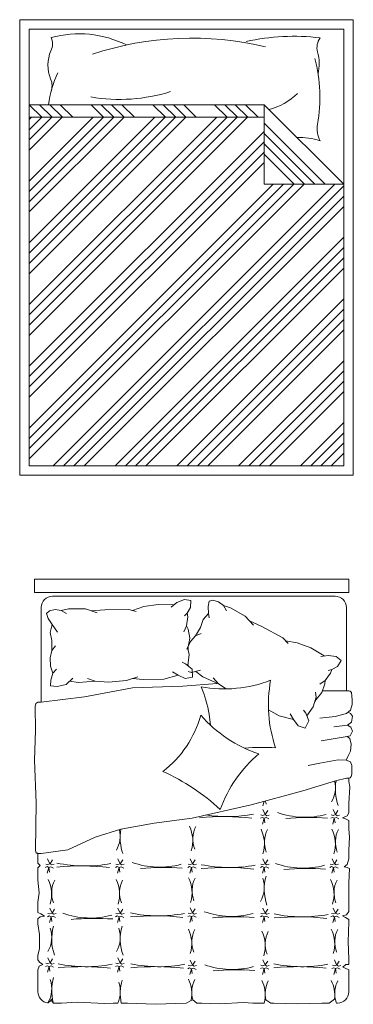
# Model space of a CAD drawing. Units: inches. Extents: x 1994 to 3075, y 3517 to 3950.
# Tile 25 of 58: x 1994.3682 to 1994.4307, y 3553.7004 to 3553.8849. Entities that reach past the tile are written whole.
import ezdxf

# ---------------------------------------------------------------- set-up
doc = ezdxf.new("R2010")
doc.units = ezdxf.units.IN
doc.layers.add('A-FURN-REFR', color=8, linetype='Continuous', lineweight=13)
doc.layers.add('A-FURN-REFR-PATT', color=8, linetype='Continuous', lineweight=13)

msp = doc.modelspace()

# ---------------------------------------------------------------- hatches: boundary and pattern name
at = {"layer": 'A-FURN-REFR-PATT'}
h = msp.add_hatch(dxfattribs=at)
h.set_pattern_fill('ANSI34', color=256, scale=0.0004294917680744, style=0)
h.set_pattern_definition([(45, (1992.977044442859, 3553.850180684118), (-0.005785419118799, 0.005785419118799), []), (45, (1992.978972916732, 3553.850180684118), (-0.005785419118799, 0.005785419118799), []), (45, (1992.980901390605, 3553.850180684118), (-0.005785419118799, 0.005785419118799), []), (45, (1992.982829868772, 3553.850180684118), (-0.005785419118799, 0.005785419118799), [])])
h.paths.add_polyline_path([(1994.370029690871, 3553.801315221915), (1994.428938814508, 3553.801315221915), (1994.428938814508, 3553.854071563733), (1994.414015178144, 3553.854071563733), (1994.414015178144, 3553.866638836461), (1994.370029690871, 3553.866638836461)])

# ---------------------------------------------------------------- linework, layer by layer
at = {"layer": 'A-FURN-REFR'}
for p, q in [((1994.368240141838, 3553.884922930949), (1994.430728363541, 3553.884922930949)), ((1994.368240141838, 3553.799525672881), (1994.368240141838, 3553.884922930949)), ((1994.430728363541, 3553.799525672881), (1994.430728363541, 3553.884922930949)), ((1994.370029690871, 3553.801315221915), (1994.370029690871, 3553.883133381916)), ((1994.370029690871, 3553.883133381916), (1994.428938814508, 3553.883133381916)), ((1994.428938814508, 3553.883133381916), (1994.428938814508, 3553.801315221915)), ((1994.370029690871, 3553.868995200097), (1994.414015178144, 3553.868995200097)), ((1994.372386054507, 3553.866638836461), (1994.370029690871, 3553.868995200097)), ((1994.370029690871, 3553.868995200097), (1994.414015178144, 3553.868995200097)), ((1994.374314532675, 3553.866638836461), (1994.371958169039, 3553.868995200097)), ((1994.376243006548, 3553.866638836461), (1994.373886642911, 3553.868995200097)), ((1994.37817148042, 3553.866638836461), (1994.375815116784, 3553.868995200097)), ((1994.383956892745, 3553.866638836461), (1994.381600529109, 3553.868995200097)), ((1994.385885370913, 3553.866638836461), (1994.383529007276, 3553.868995200097)), ((1994.387813844785, 3553.866638836461), (1994.385457481149, 3553.868995200097)), ((1994.389742318658, 3553.866638836461), (1994.387385955021, 3553.868995200097)), ((1994.395527730983, 3553.866638836461), (1994.393171367346, 3553.868995200097)), ((1994.39745620915, 3553.866638836461), (1994.395099845514, 3553.868995200097)), ((1994.399384683022, 3553.866638836461), (1994.397028319387, 3553.868995200097)), ((1994.401313156896, 3553.866638836461), (1994.398956793259, 3553.868995200097)), ((1994.407098569221, 3553.866638836461), (1994.404742205584, 3553.868995200097)), ((1994.409027047388, 3553.866638836461), (1994.406670683751, 3553.868995200097)), ((1994.41095552126, 3553.866638836461), (1994.408599157624, 3553.868995200097)), ((1994.412883995133, 3553.866638836461), (1994.410527631497, 3553.868995200097)), ((1994.428938814508, 3553.854071563733), (1994.414015178144, 3553.868995200097)), ((1994.414015178144, 3553.868995200097), (1994.414015178144, 3553.854071563733)), ((1994.414015178144, 3553.866638836461), (1994.370029690871, 3553.866638836461)), ((1994.42545126786, 3553.854071563733), (1994.414015178144, 3553.86550765345)), ((1994.423522793988, 3553.854071563733), (1994.414015178144, 3553.863579179578)), ((1994.421594320115, 3553.854071563733), (1994.414015178144, 3553.861650705704)), ((1994.419665841948, 3553.854071563733), (1994.414015178144, 3553.859722227537)), ((1994.414015178144, 3553.854071563733), (1994.428938814508, 3553.854071563733)), ((1994.428938814508, 3553.801315221915), (1994.370029690871, 3553.801315221915)), ((1994.368240141838, 3553.799525672881), (1994.430728363541, 3553.799525672881)), ((1994.374369662702, 3553.776879347694), (1994.427307661648, 3553.776879347694)), ((1994.406405658198, 3553.77509977936), (1994.407753984843, 3553.774702339899)), ((1994.406405658198, 3553.77509977936), (1994.406968598159, 3553.774142304752)), ((1994.372252142744, 3553.757002402463), (1994.372252142744, 3553.774761827737)), ((1994.403633649272, 3553.773621406152), (1994.402579506154, 3553.772507359423)), ((1994.407753984843, 3553.774702339899), (1994.410494828313, 3553.773116088013)), ((1994.410494828313, 3553.773116088013), (1994.412065912074, 3553.771412908928)), ((1994.429425181607, 3553.76268197533), (1994.429425181607, 3553.774761827737)), ((1994.402579506154, 3553.772507359423), (1994.402115540643, 3553.771021464581)), ((1994.402115540643, 3553.771021464581), (1994.401170657182, 3553.769426673137)), ((1994.399767832714, 3553.766897611043), (1994.399767832714, 3553.767096424024)), ((1994.399767832714, 3553.763831583339), (1994.399767832714, 3553.763991882089)), ((1994.429425181607, 3553.76268197533), (1994.429425181607, 3553.759155137558)), ((1994.398783393365, 3553.759994420633), (1994.405228269321, 3553.7605222814)), ((1994.393114474107, 3553.759840917956), (1994.398783393365, 3553.759994420633)), ((1994.429425181607, 3553.759155137558), (1994.429893852388, 3553.759155137558)), ((1994.371652995319, 3553.757002402463), (1994.372252613397, 3553.757002402463)), ((1994.423521127195, 3553.757099635416), (1994.42361858113, 3553.757272925152)), ((1994.403701135297, 3553.754744186191), (1994.403958917441, 3553.752696826246)), ((1994.429474495267, 3553.754878016059), (1994.427309408632, 3553.754311432808)), ((1994.430203898, 3553.755507485811), (1994.429474495267, 3553.754878016059)), ((1994.427309408632, 3553.754311432808), (1994.42447417688, 3553.754002387236)), ((1994.427103209532, 3553.752354144484), (1994.429629144984, 3553.752663190056)), ((1994.429629144984, 3553.752663190056), (1994.430247740718, 3553.75230263659)), ((1994.430557038585, 3553.751581530554), (1994.430144641951, 3553.75070590173)), ((1994.430247740718, 3553.75230263659), (1994.430557038585, 3553.751581530554)), ((1994.429216746784, 3553.750499871051), (1994.42468037598, 3553.749778765014)), ((1994.430144641951, 3553.75070590173), (1994.429216746784, 3553.750499871051)), ((1994.424459448261, 3553.74558966953), (1994.422300593145, 3553.745123270979)), ((1994.427901946281, 3553.746172667719), (1994.424459448261, 3553.74558966953)), ((1994.429418979945, 3553.7461143679), (1994.427901946281, 3553.746172667719)), ((1994.430177496776, 3553.745822868806), (1994.429418979945, 3553.7461143679)), ((1994.430462438404, 3553.745117864219), (1994.430177496776, 3553.745822868806)), ((1994.429425181607, 3553.742779105069), (1994.429893852388, 3553.742779105069)), ((1994.429893852388, 3553.742779105069), (1994.429893852388, 3553.74212236867)), ((1994.429893852388, 3553.738038066713), (1994.429893852388, 3553.736243449602)), ((1994.429893852388, 3553.734820132314), (1994.429893852388, 3553.733211165113)), ((1994.429893852388, 3553.72918874646), (1994.429893852388, 3553.727631897226)), ((1994.371652995319, 3553.726829779951), (1994.371652995319, 3553.728685223678)), ((1994.372252142744, 3553.728620422557), (1994.371652995319, 3553.728620422557)), ((1994.371652995319, 3553.723611844897), (1994.371652995319, 3553.725963413047)), ((1994.371652995319, 3553.717547275919), (1994.371652995319, 3553.719527543594)), ((1994.429893852388, 3553.718596926409), (1994.429893852388, 3553.717762449974)), ((1994.371652995319, 3553.715443241637), (1994.371652995319, 3553.716371491844)), ((1994.429893852388, 3553.716245358913), (1994.429893852388, 3553.715812175133)), ((1994.371652995319, 3553.708697955665), (1994.371652995319, 3553.709564322569)), ((1994.429893852388, 3553.708881239251), (1994.429893852388, 3553.707829221784)), ((1994.371652995319, 3553.705851321087), (1994.371652995319, 3553.706841454597)), ((1994.429893852388, 3553.706839088273), (1994.429893852388, 3553.702720755229)), ((1994.376058946635, 3553.700603235272), (1994.374596919452, 3553.700603235272)), ((1994.38661782809, 3553.700603235272), (1994.385720626736, 3553.700603235272)), ((1994.388420073799, 3553.700603235272), (1994.387271361502, 3553.700603235272)), ((1994.40235518889, 3553.700603235272), (1994.401426181978, 3553.700603235272)), ((1994.414013487327, 3553.700603235272), (1994.411893001706, 3553.700603235272)), ((1994.415856768486, 3553.700603235272), (1994.415299363426, 3553.700603235272)), ((1994.426199720931, 3553.700603235272), (1994.424837176243, 3553.700603235272)), ((1994.427560077345, 3553.700603235272), (1994.42777633243, 3553.700603235272))]:
    msp.add_line(p, q, dxfattribs=at)
msp.add_lwpolyline([(1994.370993535893, 3553.780030975446), (1994.429881082485, 3553.780030975446), (1994.429881082485, 3553.777551780742), (1994.370993535893, 3553.777551780742)], close=True, dxfattribs=at)
for points in [[(1994.389379899846, 3553.774159662139), (1994.391495423462, 3553.77490501664), (1994.394172619542, 3553.775298872562), (1994.39712136546, 3553.775228739967)], [(1994.399084448324, 3553.773206591587), (1994.399594702442, 3553.773700236123), (1994.400226090622, 3553.774741015109), (1994.400300586028, 3553.776056433098), (1994.39913322836, 3553.776216902284), (1994.397700281661, 3553.77566724495), (1994.39659355446, 3553.774828945053)], [(1994.406405658198, 3553.77509977936), (1994.405466822385, 3553.775811861941), (1994.404429321561, 3553.776144065447), (1994.403742598781, 3553.775963909912), (1994.40351379457, 3553.774962775242), (1994.403633649272, 3553.773621406152), (1994.403727248118, 3553.772789354132)], [(1994.376026324964, 3553.774197287111), (1994.374858967296, 3553.774357756296), (1994.373791819769, 3553.774138751078), (1994.373281565651, 3553.773645106542), (1994.37357287003, 3553.772660340705), (1994.374334848873, 3553.771549924374), (1994.375346156134, 3553.770146197392)], [(1994.376026324964, 3553.774197287111), (1994.377396372352, 3553.774511791517), (1994.380562898609, 3553.774472683474), (1994.382767152017, 3553.773758267566)], [(1994.376026324964, 3553.774197287111), (1994.376986329604, 3553.773638672652)], [(1994.381656957109, 3553.774118090488), (1994.384200098715, 3553.774307924899), (1994.388673773663, 3553.774348168371), (1994.39008579642, 3553.773971217203)], [(1994.398958777189, 3553.770191613156), (1994.39950861096, 3553.771304552722), (1994.39971356891, 3553.773013448286), (1994.399594702442, 3553.773700236123)], [(1994.374334848873, 3553.771549924374), (1994.373962116957, 3553.770062178177), (1994.374286068838, 3553.768539613678), (1994.374244220954, 3553.766686396676)], [(1994.399747945956, 3553.766984136998), (1994.400109875452, 3553.769027707226), (1994.399776595705, 3553.770703928636), (1994.39950861096, 3553.771304552722)], [(1994.411274619573, 3553.772270732598), (1994.413584330142, 3553.771189601976), (1994.417503409388, 3553.769031777853), (1994.418549385725, 3553.768011075178)], [(1994.402233276213, 3553.769852220113), (1994.401170657182, 3553.769426673137), (1994.400219416478, 3553.768348255874), (1994.399547527007, 3553.766963226722)], [(1994.374961828736, 3553.767578186171), (1994.374244220954, 3553.766686396676), (1994.373943716215, 3553.765280146495), (1994.374036994797, 3553.763743578786), (1994.374423846009, 3553.762456166863)], [(1994.4180264826, 3553.768521343527), (1994.420235776237, 3553.768134025673), (1994.422762338659, 3553.767165013974), (1994.42529815245, 3553.765658471747)], [(1994.399751169989, 3553.76384533263), (1994.399988868261, 3553.765935900162), (1994.399747945956, 3553.766984136998)], [(1994.426018003793, 3553.762933661213), (1994.426704726573, 3553.763113816748), (1994.427765226226, 3553.763711489248), (1994.428474948234, 3553.764821520203), (1994.427536112421, 3553.765533602784), (1994.426017694354, 3553.765756909736), (1994.424642129816, 3553.765568723605)], [(1994.396869108781, 3553.762662051774), (1994.397910668443, 3553.762031276771), (1994.39925979189, 3553.761419172675), (1994.400634503815, 3553.761656848839), (1994.400541225232, 3553.763193416547), (1994.399322563715, 3553.76419899818), (1994.398688779206, 3553.764468969762)], [(1994.375150781636, 3553.763194299799), (1994.374423846009, 3553.762456166863), (1994.374041786226, 3553.761122077577), (1994.37403019013, 3553.760041812517), (1994.375269775589, 3553.759962839385), (1994.376947387375, 3553.760296014735), (1994.378184576506, 3553.761527792171)], [(1994.389350455634, 3553.761407307046), (1994.391398246481, 3553.761250377201), (1994.395252128075, 3553.761330107378), (1994.397910668443, 3553.762031276771)], [(1994.399768886277, 3553.762736315327), (1994.400394365444, 3553.762531641508), (1994.402076517846, 3553.762998841562)], [(1994.401232126903, 3553.7627643209), (1994.402574387931, 3553.761730739291), (1994.405449609264, 3553.760421493173)], [(1994.424430587178, 3553.760367341538), (1994.425455373825, 3553.761067887029), (1994.426471684252, 3553.762456931638), (1994.426704726573, 3553.763113816748)], [(1994.377563544014, 3553.760909476191), (1994.379240127958, 3553.760666531976), (1994.382387998502, 3553.760934737404)], [(1994.380966647265, 3553.761465345445), (1994.382387998502, 3553.760934737404), (1994.384867168785, 3553.760776791455), (1994.388245712014, 3553.761059000053), (1994.390366014664, 3553.761727495645)], [(1994.404470821382, 3553.761580699158), (1994.405449609264, 3553.760421493173), (1994.406887043621, 3553.759488094975)], [(1994.423546206662, 3553.757184801398), (1994.424863387386, 3553.758788611605), (1994.425394541905, 3553.760413009488), (1994.425455373825, 3553.761067887029)], [(1994.372252613397, 3553.757002402463), (1994.380392096975, 3553.757998261552), (1994.389362140071, 3553.759658026504), (1994.393114474107, 3553.759840917956)], [(1994.422010441024, 3553.754447370638), (1994.423242376189, 3553.756153040251), (1994.423771411884, 3553.75794956339), (1994.423622200712, 3553.75887743124)], [(1994.42498323605, 3553.759155137558), (1994.429425652259, 3553.759155137558)], [(1994.429893852388, 3553.759155137558), (1994.430137944852, 3553.759073556183), (1994.430412507876, 3553.758799217356), (1994.430490954223, 3553.757420990779), (1994.430542340634, 3553.756552727357)], [(1994.371652995319, 3553.757002402463), (1994.371239196245, 3553.756726399039), (1994.37112370645, 3553.756207118058), (1994.371181451348, 3553.751706682294), (1994.371008216138, 3553.746109986878), (1994.371296941142, 3553.738147677905), (1994.371181451348, 3553.729262202644), (1994.371296941142, 3553.728685223678), (1994.371652995319, 3553.728685223678)], [(1994.430542340634, 3553.756552727357), (1994.430203898, 3553.755507485811)], [(1994.414840307951, 3553.755539734691), (1994.416856067451, 3553.754460380967), (1994.419517007735, 3553.753768375036)], [(1994.418918354215, 3553.754828722901), (1994.419517007735, 3553.753768375036), (1994.42039289265, 3553.752573539853), (1994.421707625421, 3553.752106848761), (1994.422379514892, 3553.753491877914), (1994.421810217842, 3553.754965727019), (1994.421390131811, 3553.755511707957)], [(1994.429745537723, 3553.755111923912), (1994.430196191334, 3553.754878016059), (1994.430557038585, 3553.754362940702), (1994.430402388869, 3553.7532812812), (1994.429629144984, 3553.752663190056)], [(1994.429610551763, 3553.750587311863), (1994.430060801397, 3553.750195353428), (1994.430352539844, 3553.749145957585), (1994.430235844465, 3553.747805061751), (1994.429710716826, 3553.74681396483), (1994.429418979945, 3553.7461143679)], [(1994.429893852388, 3553.742779105069), (1994.430158810292, 3553.74282672715), (1994.430322240182, 3553.743048811095), (1994.430479132875, 3553.74351257445), (1994.430462438404, 3553.745117864219)], [(1994.372252142744, 3553.728620422557), (1994.377258563176, 3553.729322034035), (1994.382359210027, 3553.731683821727), (1994.387211044382, 3553.733175476649), (1994.39343134463, 3553.734294218187), (1994.400522487398, 3553.735288655111), (1994.411594622811, 3553.737774746955), (1994.421298292331, 3553.740385143414), (1994.427394186735, 3553.742249712182), (1994.429425181607, 3553.742779105069)], [(1994.429893852388, 3553.738038066713), (1994.430062065296, 3553.741133415707), (1994.429893852388, 3553.74212236867)], [(1994.413431986664, 3553.735883925484), (1994.413793317279, 3553.735789742057), (1994.414233198661, 3553.735946714436), (1994.414688790035, 3553.73666878738)], [(1994.414987280684, 3553.735836833771), (1994.414547399302, 3553.735711255868), (1994.414216404339, 3553.735920096887), (1994.413793317279, 3553.736888548247)], [(1994.426594833989, 3553.735883925484), (1994.426956164605, 3553.735789742057), (1994.427396045987, 3553.735946714436), (1994.427851637361, 3553.73666878738)], [(1994.42815012801, 3553.735836833771), (1994.427710246627, 3553.735711255868), (1994.427379251665, 3553.735920096887), (1994.426956164605, 3553.736888548247)], [(1994.429893852388, 3553.734820132314), (1994.429256925668, 3553.735130729378), (1994.428699520608, 3553.735316379942), (1994.429566595019, 3553.735687679764), (1994.429893852388, 3553.736243449602)], [(1994.413337726714, 3553.735256036432), (1994.413683347338, 3553.735397311573), (1994.41401325797, 3553.735240339193), (1994.414154648704, 3553.734376991573)], [(1994.414877309934, 3553.735130458528), (1994.414390299386, 3553.735381614335), (1994.41401325797, 3553.735240339193), (1994.413714767321, 3553.734157230241)], [(1994.42650057404, 3553.735256036432), (1994.426846194664, 3553.735397311573), (1994.427176105296, 3553.735240339193), (1994.427317496029, 3553.734376991573)], [(1994.42804015726, 3553.735130458528), (1994.427553146712, 3553.735381614335), (1994.427176105296, 3553.735240339193), (1994.426877614647, 3553.734157230241)], [(1994.429893852388, 3553.72918874646), (1994.430000131654, 3553.731789028371), (1994.429893852388, 3553.733211165113)], [(1994.373116485853, 3553.726657353991), (1994.373477816468, 3553.726563170563), (1994.373917697851, 3553.726720142942), (1994.374373289225, 3553.727442215887)], [(1994.374671779874, 3553.726610262277), (1994.374231898491, 3553.726484684374), (1994.373900903528, 3553.726693525393), (1994.373477816468, 3553.727661976754)], [(1994.386273964593, 3553.726657353991), (1994.386635295209, 3553.726563170563), (1994.387075176591, 3553.726720142942), (1994.387530767965, 3553.727442215887)], [(1994.387829258614, 3553.726610262277), (1994.387389377232, 3553.726484684374), (1994.387058382269, 3553.726693525393), (1994.386635295209, 3553.727661976754)], [(1994.399821387241, 3553.726657353991), (1994.400182717856, 3553.726563170563), (1994.400622599238, 3553.726720142942), (1994.401078190612, 3553.727442215887)], [(1994.401376681262, 3553.726610262277), (1994.400936799879, 3553.726484684374), (1994.400605804916, 3553.726693525393), (1994.400182717856, 3553.727661976754)], [(1994.413431986664, 3553.726657353991), (1994.413793317279, 3553.726563170563), (1994.414233198661, 3553.726720142942), (1994.414688790035, 3553.727442215887)], [(1994.414987280684, 3553.726610262277), (1994.414547399302, 3553.726484684374), (1994.414216404339, 3553.726693525393), (1994.413793317279, 3553.727661976754)], [(1994.426418264744, 3553.726657353991), (1994.426779595359, 3553.726563170563), (1994.427219476742, 3553.726720142942), (1994.427675068116, 3553.727442215887)], [(1994.427973558765, 3553.726610262277), (1994.427533677383, 3553.726484684374), (1994.42720268242, 3553.726693525393), (1994.426779595359, 3553.727661976754)], [(1994.429893852388, 3553.718596926409), (1994.429871042563, 3553.723146302614), (1994.429994909847, 3553.725807286627), (1994.429561373212, 3553.725992936538), (1994.429003968152, 3553.726116703799), (1994.429561373212, 3553.726549886925), (1994.429893852388, 3553.727631897226)], [(1994.371652995319, 3553.726829779951), (1994.372103251061, 3553.726371100662), (1994.371652995319, 3553.725963413047)], [(1994.373022225904, 3553.726029464939), (1994.373367846527, 3553.72617074008), (1994.37369775716, 3553.7260137677), (1994.373839147893, 3553.725150420079)], [(1994.374561809123, 3553.725903887035), (1994.374074798576, 3553.726155042841), (1994.37369775716, 3553.7260137677), (1994.37339926651, 3553.724930658748)], [(1994.386179704644, 3553.726029464939), (1994.386525325268, 3553.72617074008), (1994.3868552359, 3553.7260137677), (1994.386996626634, 3553.725150420079)], [(1994.387719287864, 3553.725903887035), (1994.387232277317, 3553.726155042841), (1994.3868552359, 3553.7260137677), (1994.386556745251, 3553.724930658748)], [(1994.399727127292, 3553.726029464939), (1994.400072747915, 3553.72617074008), (1994.400402658547, 3553.7260137677), (1994.400544049281, 3553.725150420079)], [(1994.401266710511, 3553.725903887035), (1994.400779699964, 3553.726155042841), (1994.400402658547, 3553.7260137677), (1994.400104167898, 3553.724930658748)], [(1994.413337726714, 3553.726029464939), (1994.413683347338, 3553.72617074008), (1994.41401325797, 3553.7260137677), (1994.414154648704, 3553.725150420079)], [(1994.414877309934, 3553.725903887035), (1994.414390299386, 3553.726155042841), (1994.41401325797, 3553.7260137677), (1994.413714767321, 3553.724930658748)], [(1994.426324004795, 3553.726029464939), (1994.426669625418, 3553.72617074008), (1994.426999536051, 3553.7260137677), (1994.427140926784, 3553.725150420079)], [(1994.427863588014, 3553.725903887035), (1994.427376577467, 3553.726155042841), (1994.426999536051, 3553.7260137677), (1994.426701045401, 3553.724930658748)], [(1994.371652995319, 3553.723611844897), (1994.371855516493, 3553.72123478189), (1994.371652995319, 3553.719527543594)], [(1994.373521320336, 3553.717410971881), (1994.373882650952, 3553.717316788453), (1994.374322532334, 3553.717473760833), (1994.374778123708, 3553.718195833777)], [(1994.375076614357, 3553.717363880168), (1994.374636732975, 3553.717238302264), (1994.374305738012, 3553.717447143283), (1994.373882650952, 3553.718415594644)], [(1994.386273964593, 3553.717410971881), (1994.386635295209, 3553.717316788453), (1994.387075176591, 3553.717473760833), (1994.387530767965, 3553.718195833777)], [(1994.387829258614, 3553.717363880168), (1994.387389377232, 3553.717238302264), (1994.387058382269, 3553.717447143283), (1994.386635295209, 3553.718415594644)], [(1994.399821387241, 3553.717456636363), (1994.400182717856, 3553.717362452935), (1994.400622599238, 3553.717519425314), (1994.401078190612, 3553.718241498258)], [(1994.401376681262, 3553.717409544649), (1994.400936799879, 3553.717283966745), (1994.400605804916, 3553.717492807765), (1994.400182717856, 3553.718461259125)], [(1994.413431986664, 3553.717410971881), (1994.413793317279, 3553.717316788453), (1994.414233198661, 3553.717473760833), (1994.414688790035, 3553.718195833777)], [(1994.414987280684, 3553.717363880168), (1994.414547399302, 3553.717238302264), (1994.414216404339, 3553.717447143283), (1994.413793317279, 3553.718415594644)], [(1994.426624308092, 3553.717410971881), (1994.426985638708, 3553.717316788453), (1994.42742552009, 3553.717473760833), (1994.427881111464, 3553.718195833777)], [(1994.428179602113, 3553.717363880168), (1994.427739720731, 3553.717238302264), (1994.427408725768, 3553.717447143283), (1994.426985638708, 3553.718415594644)], [(1994.429893852388, 3553.716245358913), (1994.429251703861, 3553.716648549203), (1994.428694298801, 3553.716957966374), (1994.429437504787, 3553.717143616285), (1994.429893852388, 3553.717762449974)], [(1994.371652995319, 3553.717547275919), (1994.372227119486, 3553.717336129844), (1994.37290839183, 3553.716902946719), (1994.372103251061, 3553.716779180112), (1994.371652995319, 3553.716371491844)], [(1994.373427060387, 3553.716783082828), (1994.373772681011, 3553.716924357969), (1994.374102591643, 3553.716767385591), (1994.374243982376, 3553.715904037969)], [(1994.374966643607, 3553.716657504925), (1994.374479633059, 3553.716908660732), (1994.374102591643, 3553.716767385591), (1994.373804100994, 3553.715684276638)], [(1994.386179704644, 3553.716783082828), (1994.386525325268, 3553.716924357969), (1994.3868552359, 3553.716767385591), (1994.386996626634, 3553.715904037969)], [(1994.387719287864, 3553.716657504925), (1994.387232277317, 3553.716908660732), (1994.3868552359, 3553.716767385591), (1994.386556745251, 3553.715684276638)], [(1994.399727127292, 3553.716828747309), (1994.400072747915, 3553.716970022451), (1994.400402658547, 3553.716813050072), (1994.400544049281, 3553.71594970245)], [(1994.401266710511, 3553.716703169406), (1994.400779699964, 3553.716954325213), (1994.400402658547, 3553.716813050072), (1994.400104167898, 3553.715729941119)], [(1994.413337726714, 3553.716783082828), (1994.413683347338, 3553.716924357969), (1994.41401325797, 3553.716767385591), (1994.414154648704, 3553.715904037969)], [(1994.414877309934, 3553.716657504925), (1994.414390299386, 3553.716908660732), (1994.41401325797, 3553.716767385591), (1994.413714767321, 3553.715684276638)], [(1994.426530048143, 3553.716783082828), (1994.426875668767, 3553.716924357969), (1994.427205579398, 3553.716767385591), (1994.427346970132, 3553.715904037969)], [(1994.428069631363, 3553.716657504925), (1994.427582620815, 3553.716908660732), (1994.427205579398, 3553.716767385591), (1994.42690708875, 3553.715684276638)], [(1994.429893852388, 3553.708881239251), (1994.429747174138, 3553.712069180818), (1994.429893852388, 3553.715812175133)], [(1994.371652995319, 3553.715443241637), (1994.371917450135, 3553.713437478451), (1994.371917450135, 3553.710776493783), (1994.371652995319, 3553.709564322569)], [(1994.371652995319, 3553.708697955665), (1994.371979383777, 3553.708239276376), (1994.372598722479, 3553.707806092597), (1994.371855516493, 3553.707496676079), (1994.371652995319, 3553.706841454597)], [(1994.373149717343, 3553.708093952432), (1994.373511047959, 3553.707999769005), (1994.373950929341, 3553.708156741385), (1994.374406520715, 3553.708878814328)], [(1994.374705011364, 3553.708046860719), (1994.374265129982, 3553.707921282815), (1994.373934135019, 3553.708130123836), (1994.373511047959, 3553.709098575196)], [(1994.386273964593, 3553.708093952432), (1994.386635295209, 3553.707999769005), (1994.387075176591, 3553.708156741385), (1994.387530767965, 3553.708878814328)], [(1994.387829258614, 3553.708046860719), (1994.387389377232, 3553.707921282815), (1994.387058382269, 3553.708130123836), (1994.386635295209, 3553.709098575196)], [(1994.399821387241, 3553.707664168773), (1994.400182717856, 3553.707569985346), (1994.400622599238, 3553.707726957725), (1994.401078190612, 3553.708449030669)], [(1994.401376681262, 3553.70761707706), (1994.400936799879, 3553.707491499157), (1994.400605804916, 3553.707700340176), (1994.400182717856, 3553.708668791536)], [(1994.413431986664, 3553.707700808332), (1994.413793317279, 3553.707606624905), (1994.414233198661, 3553.707763597284), (1994.414688790035, 3553.708485670228)], [(1994.414987280684, 3553.707653716618), (1994.414547399302, 3553.707528138715), (1994.414216404339, 3553.707736979735), (1994.413793317279, 3553.708705431095)], [(1994.42682114754, 3553.707700808332), (1994.427182478155, 3553.707606624905), (1994.427622359538, 3553.707763597284), (1994.428077950912, 3553.708485670228)], [(1994.428376441561, 3553.707653716618), (1994.427936560178, 3553.707528138715), (1994.427605565215, 3553.707736979735), (1994.427182478155, 3553.708705431095)], [(1994.373055457394, 3553.707466063379), (1994.373401078018, 3553.707607338521), (1994.37373098865, 3553.707450366142), (1994.373872379383, 3553.70658701852)], [(1994.374595040614, 3553.707340485476), (1994.374108030066, 3553.707591641283), (1994.37373098865, 3553.707450366142), (1994.373432498001, 3553.70636725719)], [(1994.386179704644, 3553.707466063379), (1994.386525325268, 3553.707607338521), (1994.3868552359, 3553.707450366142), (1994.386996626634, 3553.70658701852)], [(1994.387719287864, 3553.707340485476), (1994.387232277317, 3553.707591641283), (1994.3868552359, 3553.707450366142), (1994.386556745251, 3553.70636725719)], [(1994.399727127292, 3553.70703627972), (1994.400072747915, 3553.707177554862), (1994.400402658547, 3553.707020582483), (1994.400544049281, 3553.706157234861)], [(1994.401266710511, 3553.706910701817), (1994.400779699964, 3553.707161857624), (1994.400402658547, 3553.707020582483), (1994.400104167898, 3553.70593747353)], [(1994.413337726714, 3553.707072919279), (1994.413683347338, 3553.707214194421), (1994.41401325797, 3553.707057222041), (1994.414154648704, 3553.70619387442)], [(1994.414877309934, 3553.706947341376), (1994.414390299386, 3553.707198497182), (1994.41401325797, 3553.707057222041), (1994.413714767321, 3553.705974113089)], [(1994.426726887591, 3553.707072919279), (1994.427072508215, 3553.707214194421), (1994.427402418846, 3553.707057222041), (1994.42754380958, 3553.70619387442)], [(1994.428266470811, 3553.706947341376), (1994.427779460263, 3553.707198497182), (1994.427402418846, 3553.707057222041), (1994.427103928198, 3553.705974113089)], [(1994.429893852388, 3553.706839088273), (1994.429189770219, 3553.707118511957), (1994.428756232443, 3553.707304162521), (1994.429313637503, 3553.707799228949), (1994.429893852388, 3553.707829221784)], [(1994.371652995319, 3553.705851321087), (1994.371607780784, 3553.704154974419), (1994.371652995319, 3553.702720755229)], [(1994.373560720093, 3553.700670936779), (1994.373993773372, 3553.701019972497), (1994.374120358825, 3553.701369660978), (1994.374269284163, 3553.70096789179), (1994.374596919452, 3553.700603235272)], [(1994.388420073799, 3553.700603235272), (1994.393663281398, 3553.700368966602), (1994.399444298588, 3553.700603235272), (1994.400359070559, 3553.7011101967), (1994.40067589277, 3553.701201830482), (1994.401426181978, 3553.700603235272)], [(1994.414013487327, 3553.700603235272), (1994.414159659663, 3553.701146974472), (1994.41436255302, 3553.701195062122), (1994.415299363426, 3553.700603235272)], [(1994.426199720931, 3553.700603235272), (1994.42720722783, 3553.701356324601), (1994.427341187654, 3553.701382813724), (1994.427569926205, 3553.700603235272)], [(1994.376058946635, 3553.700603235272), (1994.378984960322, 3553.700740267076), (1994.384187403365, 3553.700492733208), (1994.385720626736, 3553.700603235272)], [(1994.40235518889, 3553.700603235272), (1994.405740382665, 3553.700430849904), (1994.410137684939, 3553.700678383119), (1994.411893001706, 3553.700603235272)], [(1994.415856768486, 3553.700603235272), (1994.420333229747, 3553.700435109289), (1994.424837176243, 3553.700603235272)]]:
    msp.add_lwpolyline(points, dxfattribs=at)
for centre, radius, start, end in [((1994.379382741791, 3553.8625259185), 0.0197486987265365, 63.38196750841395, 105.3587807882128), ((1994.371176451099, 3553.880384435683), 0.0032028341489732, 335.7877323280015, 21.71237864400314), ((1994.400441073425, 3553.822794491352), 0.0586716085832465, 76.33335198625635, 108.4694926903225), ((1994.41955592446, 3553.84034223252), 0.0414680575843914, 83.14136388124066, 102.4247502365447), ((1994.427034094371, 3553.879703646134), 0.0031075126812102, 144.3787648229011, 195.1987658355305), ((1994.380095490524, 3553.876373764836), 0.0065764677133891, 155.7877323280015, 202.8808293159797), ((1994.4157396765, 3553.876635281956), 0.0085962787467616, 347.311957921453, 15.19876583553051), ((1994.394600074051, 3553.870321435996), 0.0298558147000044, 350.3711224665587, 14.25995084780135), ((1994.393362632327, 3553.866610535198), 0.0198519972069101, 155.1179531461462, 173.1008468379609), ((1994.370959122235, 3553.872518013683), 0.0033401870886801, 339.0160855821216, 22.88082931597971), ((1994.38693399472, 3553.902211153669), 0.0322267158934928, 260.4320326468418, 287.2701993260345), ((1994.412168401375, 3553.879202216185), 0.0114567055564695, 283.9361364524131, 315.0098308273483), ((1994.428960978581, 3553.864491908892), 0.004996088352876, 170.3711224665586, 206.9649370961853), ((1994.420397575666, 3553.849300124312), 0.0135641447689492, 72.35976010254194, 91.05260058094025), ((1994.374369662702, 3553.774761827737), 0.0021175199578634, 90, 180), ((1994.427307661648, 3553.774761827737), 0.0021175199578634, 0, 90), ((1994.406479084909, 3553.784127917182), 0.0246431992375616, 260.0745918606295, 290.8409915293051), ((1994.43953766185, 3553.756527947085), 0.0247171166068797, 169.3471826619405, 199.0940702927494), ((1994.383882284237, 3553.751809397177), 0.0200349655328587, 8.423186569474346, 23.67235024141385), ((1994.38284742713, 3553.759879579041), 0.0200349655328587, 307.5937276079389, 344.5933654173315), ((1994.420762127194, 3553.770722902098), 0.0246431992375616, 220.9956070369567, 251.7620067056939), ((1994.429025986335, 3553.728457827973), 0.0247171166068797, 130.268197838044, 160.0150854690268), ((1994.413705526148, 3553.707646392015), 0.0408710896652553, 86.52841791930182, 94.68904240848443), ((1994.378158577626, 3553.706796517021), 0.0408710896652553, 47.44943309542468, 65.55793652235621), ((1994.422023465027, 3553.740998955435), 0.0053493603954956, 330.0061435674863, 12.98914022263098), ((1994.436264326926, 3553.740659490975), 0.0089008848270733, 169.506879604364, 199.7292868004655), ((1994.407844211258, 3553.739439126662), 0.006239009817234, 342.64426438976, 350.6149706842582), ((1994.419240504231, 3553.739755354231), 0.0051620947334588, 194.239775801134, 201.5194296612977), ((1994.421652081081, 3553.750786268621), 0.0153539547651982, 250.4133200326824, 285.1509893024539), ((1994.406403853355, 3553.689567699051), 0.0459976774432946, 83.32535582969805, 95.58421926114355), ((1994.407217191363, 3553.761754168354), 0.0261988152598324, 261.0363713148148, 280.5874491149217), ((1994.42242482961, 3553.685434831458), 0.0499412040235263, 86.03505303173033, 95.0058073178226), ((1994.381715707367, 3553.731951385787), 0.0053493603954956, 330.0061435674863, 12.31935640363241), ((1994.395956569265, 3553.731611921327), 0.0089008848270733, 169.9188183421145, 199.7292868004655), ((1994.394427975574, 3553.731022942742), 0.006239009817234, 342.64426438976, 26.16029174252129), ((1994.405824268547, 3553.731339170312), 0.0051620947334588, 152.7510931195746, 201.5194296612977), ((1994.407844211258, 3553.73045504817), 0.006239009817234, 342.64426438976, 26.16029174252129), ((1994.419240504231, 3553.73077127574), 0.0051620947334588, 152.7510931195746, 201.5194296612977), ((1994.421136928127, 3553.73045504817), 0.006239009817234, 342.64426438976, 26.16029174252129), ((1994.4325332211, 3553.73077127574), 0.0051620947334588, 152.7510931195746, 201.5194296612977), ((1994.394448995012, 3553.74142579604), 0.0153539547651982, 250.4133200326824, 285.1509893024539), ((1994.380509805366, 3553.752500162354), 0.0261988152598324, 258.3524138495688, 280.5874491149217), ((1994.379696467358, 3553.680313693052), 0.0459976774432946, 83.32535582969805, 95.58421926114355), ((1994.395221743542, 3553.676074358878), 0.0499412040235263, 86.03505303173033, 95.0058073178226), ((1994.407548683587, 3553.752200820953), 0.0261988152598324, 258.3524138495688, 280.5874491149217), ((1994.406735345578, 3553.68001435165), 0.0459976774432946, 83.32535582969805, 95.58421926114355), ((1994.421319533333, 3553.741242154821), 0.0153539547651982, 250.4133200326824, 285.1509893024539), ((1994.422092281863, 3553.675890717658), 0.0499412040235263, 86.03505303173033, 95.0058073178226), ((1994.367987519254, 3553.720987924352), 0.006239009817234, 342.64426438976, 26.16029174252129), ((1994.379383812226, 3553.721304151922), 0.0051620947334588, 152.7510931195746, 201.5194296612977), ((1994.380718896311, 3553.720987924352), 0.006239009817234, 342.64426438976, 26.16029174252129), ((1994.392115189284, 3553.721304151922), 0.0051620947334588, 152.7510931195746, 201.5194296612977), ((1994.394285491824, 3553.721342606926), 0.006239009817234, 342.64426438976, 26.16029174252129), ((1994.405681784797, 3553.721658834496), 0.0051620947334588, 152.7510931195746, 201.5194296612977), ((1994.408698980103, 3553.722302087101), 0.0053493603954956, 330.0061435674863, 18.99185374207843), ((1994.422939842001, 3553.721962622642), 0.0089008848270733, 163.9853342830063, 199.7292868004655), ((1994.420878515105, 3553.720987924352), 0.006239009817234, 342.64426438976, 26.16029174252129), ((1994.432274808078, 3553.721304151922), 0.0051620947334588, 152.7510931195746, 201.5194296612977), ((1994.407946302022, 3553.732198680241), 0.0153539547651982, 250.4133200326824, 285.1509893024539), ((1994.381453738785, 3553.731889492967), 0.0153539547651982, 250.4133200326824, 285.1509893024539), ((1994.382226487315, 3553.666538055805), 0.0499412040235263, 86.03505303173033, 95.0058073178226), ((1994.394274261562, 3553.743144055851), 0.0261988152598324, 258.3524138495688, 280.5874491149217), ((1994.393460923554, 3553.670957586547), 0.0459976774432946, 83.32535582969805, 95.58421926114355), ((1994.408719050552, 3553.666847243079), 0.0499412040235263, 86.03505303173033, 95.0058073178226), ((1994.421215223187, 3553.742958695476), 0.0261988152598324, 258.3524138495688, 280.5874491149217), ((1994.420401885178, 3553.670772226174), 0.0459976774432946, 83.32535582969805, 95.58421926114355), ((1994.368887988412, 3553.712917498621), 0.0053493603954956, 330.0061435674863, 18.99185374207843), ((1994.383128850311, 3553.712578034161), 0.0089008848270733, 163.9853342830063, 199.7292868004655), ((1994.381737023083, 3553.712917498621), 0.0053493603954956, 330.0061435674863, 18.99185374207843), ((1994.395977884981, 3553.712578034161), 0.0089008848270733, 163.9853342830063, 199.7292868004655), ((1994.394238449106, 3553.711725770853), 0.006239009817234, 342.64426438976, 26.16029174252129), ((1994.405634742079, 3553.712041998422), 0.0051620947334588, 152.7510931195746, 201.5194296612977), ((1994.407989204062, 3553.711340929833), 0.006239009817234, 342.64426438976, 26.16029174252129), ((1994.419385497035, 3553.711657157403), 0.0051620947334588, 152.7510931195746, 201.5194296612977), ((1994.421008934632, 3553.711725770853), 0.006239009817234, 342.64426438976, 26.16029174252129), ((1994.432405227605, 3553.712041998422), 0.0051620947334588, 152.7510931195746, 201.5194296612977), ((1994.380715920492, 3553.733618071166), 0.0261988152598324, 258.3524138495688, 280.5874491149217), ((1994.379902582484, 3553.661431601863), 0.0459976774432946, 83.32535582969805, 95.58421926114355), ((1994.39437493898, 3553.733618071166), 0.0261988152598324, 258.3524138495688, 280.5874491149217), ((1994.393561600971, 3553.661431601863), 0.0459976774432946, 83.32535582969805, 95.58421926114355), ((1994.408035759972, 3553.722249834382), 0.0153539547651982, 250.4133200326824, 285.1509893024539), ((1994.408808508502, 3553.65689839722), 0.0499412040235263, 86.03505303173033, 95.0058073178226), ((1994.42113209143, 3553.733618071166), 0.0261988152598324, 258.3524138495688, 280.5874491149217), ((1994.420318753421, 3553.661431601863), 0.0459976774432946, 83.32535582969805, 95.58421926114355), ((1994.368887988412, 3553.703275017286), 0.0053493603954956, 330.0061435674863, 18.99185374207843), ((1994.383128850311, 3553.702935552826), 0.0089008848270733, 163.9853342830063, 194.5805863570836), ((1994.395977884981, 3553.702453154086), 0.0089008848270733, 163.9853342830063, 191.9955302954556), ((1994.394238449106, 3553.702319839842), 0.006239009817234, 348.8204723522059, 26.16029174252129), ((1994.405634742079, 3553.702636067412), 0.0051620947334588, 152.7510931195746, 196.1313374827651), ((1994.407989204062, 3553.702069319943), 0.006239009817234, 351.4985040698443, 26.16029174252129), ((1994.419385497035, 3553.702385547512), 0.0051620947334588, 152.7510931195746, 193.3336118673377), ((1994.421008934632, 3553.702067945935), 0.006239009817234, 353.4505908868089, 26.16029174252129), ((1994.432405227605, 3553.702384173504), 0.0051620947334588, 152.7510931195746, 191.1853325139393), ((1994.381737023083, 3553.702792618546), 0.0053493603954956, 335.8404210583651, 18.99185374207843), ((1994.373770515277, 3553.702720755229), 0.0021175199578634, 180, 263.4835895039438), ((1994.42777633243, 3553.702720755229), 0.0021175199578634, 270, 0)]:
    msp.add_arc(centre, radius, start, end, dxfattribs=at)

doc.saveas('drawing.dxf')
